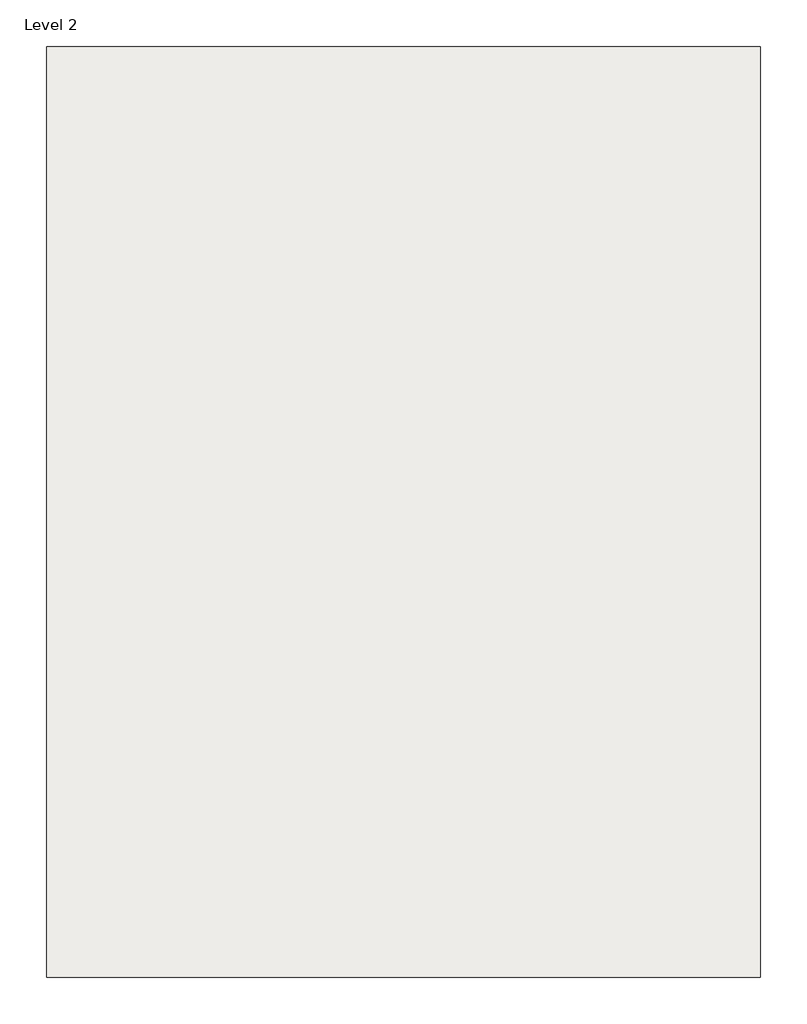
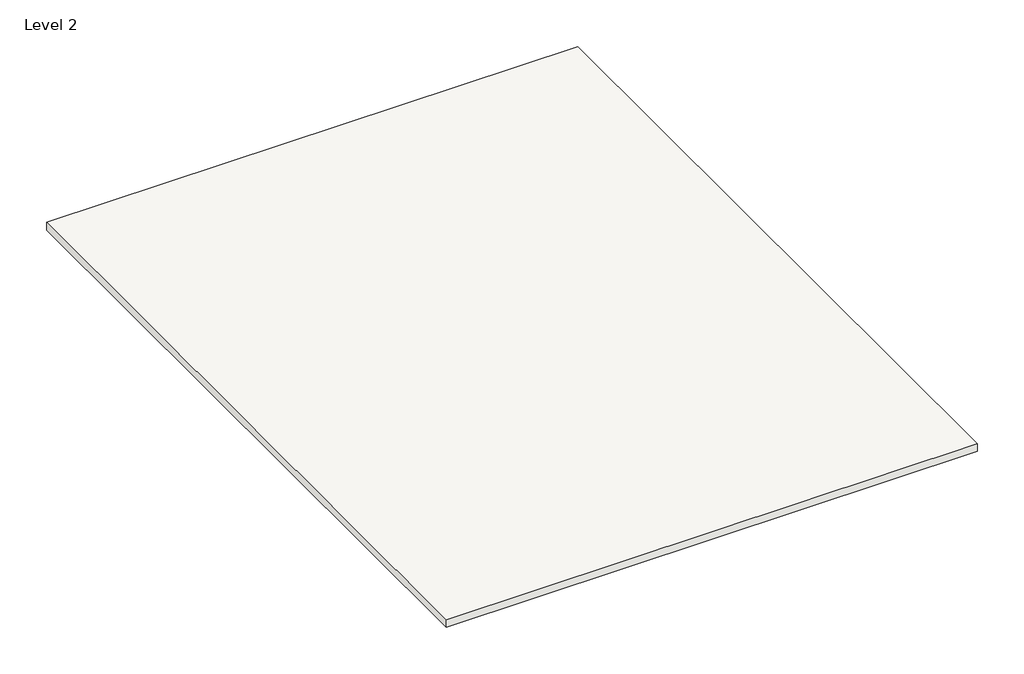
# One storey, incomplete: 1 roof.
"""IFC4 building model written with IfcOpenShell, lengths in millimetres."""

from ifc_helpers import new_model, si_unit, frame, origin, place, context, project, spatial, polyline, outline, extrude, element, save

model = new_model("IFC4")

# Units and contexts
model_context = context("Model", 3, world=origin())
ifc_project = project(units=[si_unit("LENGTHUNIT", "METRE", prefix="MILLI")], contexts=[model_context])

# Site, building, storey
site = spatial("IfcSite", under=ifc_project)
building = spatial("IfcBuilding", under=site)
storey = spatial("IfcBuildingStorey", under=building, Name="Level 2", Elevation=3048.0)

# Roof
placement = place(None, origin())
element("IfcRoof", 1, ObjectType="ROOF 6\"", at=placement, inside=storey, context=model_context, shape_type="SweptSolid", body=[
    extrude(outline(polyline([(-6271.8410855, 6364.6803617), (3761.1589145, 6364.6803617), (3761.1589145, -6716.3196383), (-6271.8410855, -6716.3196383), (-6271.8410855, 6364.6803617)])), frame((0.0, 0.0, 3048.0), z_axis=(0.0, 0.0, 1.0), x_axis=(1.0, 0.0, 0.0)), (0.0, 0.0, 1.0), 152.4),
])

save(model, "model.ifc")

# Revit data of these elements
# Type "ROOF 6\""
#   Assembly Code = "B1020"
#   Layers, outside or top first: 0' - 6" no material (function 1)
# Element 1 (IfcRoof, "ROOF 6\"")
#   built-in parameter 1001705 = 10.5 (stored number, unit not read)
#   built-in parameter 1001710 = 33615
#   Phase Created = New Construction
#   Materials on its faces: "Default Roof", "Oak Flooring"
# Materials
#   "Default Roof": colour RGB 88 101 114, transparency 0, Cost = 0
#   "Oak Flooring": class "Wood", colour RGB 216 169 114, transparency 0, Description = "Quercus Rubra", Cost = 0
